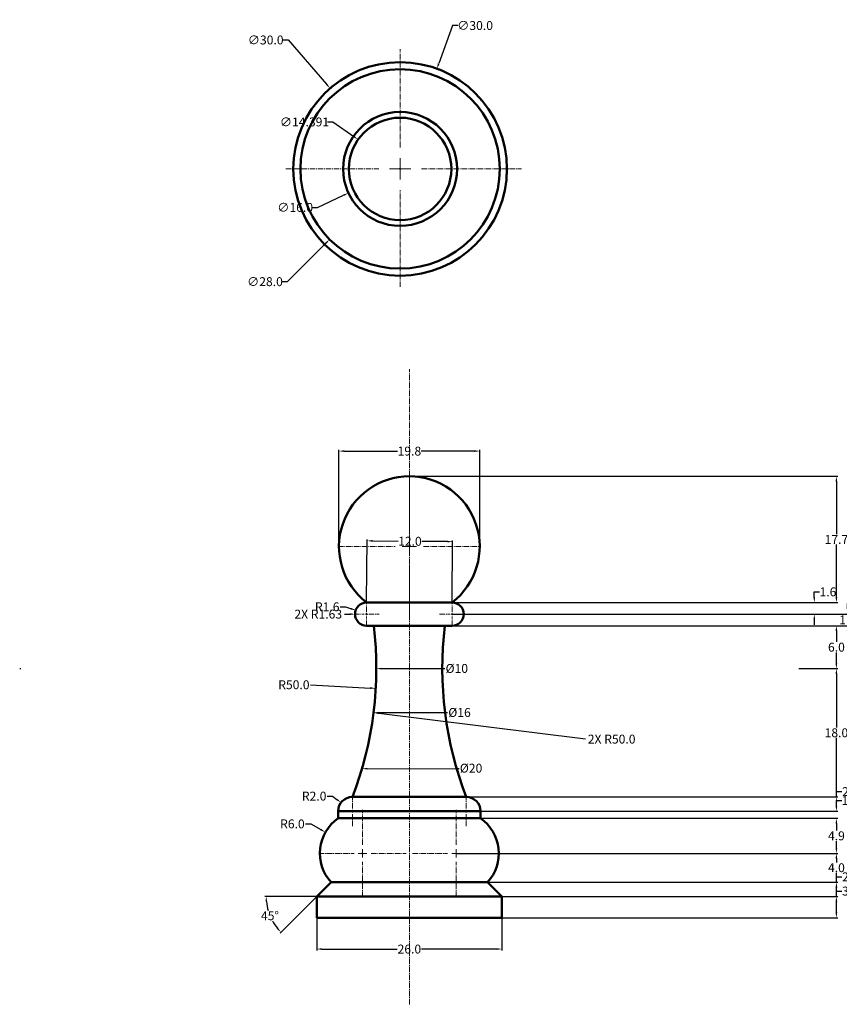
# Model space of a CAD drawing. Units: millimetres. Extents: x 10 to 184, y 6 to 153.
# Tile 1 of 2: x 10 to 125, y 14 to 153. Entities that reach past the tile are written whole.
import ezdxf
from ezdxf import colors
from ezdxf.entities.mleader import LeaderData, LeaderLine
from ezdxf.math import Vec2, Vec3

# ---------------------------------------------------------------- set-up
doc = ezdxf.new("R2010")
doc.units = ezdxf.units.MM
doc.header["$MEASUREMENT"] = 0
doc.linetypes.add('CENTER2', pattern=[1.125, 0.75, -0.125, 0.125, -0.125])
for name, color, linetype, lineweight in [('M-CNTR', 4, 'CENTER2', 18), ('M-DIMS', 2, 'Continuous', 25), ('M-OUTL', 7, 'Continuous', 50)]:
    doc.layers.add(name, color=color, linetype=linetype, lineweight=lineweight)
doc.styles.get("Standard").update_dxf_attribs({"font": 'arial.ttf'})
doc.dimstyles.get("Standard").update_dxf_attribs({"dimtxt": 1.25, "dimasz": 0.75, "dimexe": 0.18, "dimexo": 0.0625, "dimgap": 0.09, "dimtad": 0, "dimtih": 1, "dimtoh": 1, "dimdec": 1, "dimzin": 0, "dimdsep": 46, "dimtxsty": 'Standard', "dimcen": 0.09, "dimadec": 0, "dimazin": 0, "dimtfac": 1, "dimtdec": 1, "dimtofl": 0, "dimtmove": 0, "dimatfit": 3, "dimfxl": 1, "dimtolj": 1, "dimtzin": 0, "dimarcsym": 0})

# ---------------------------------------------------------------- blocks, each defined once
blk = doc.blocks.new('*U1')
at = {"layer": 'M-CNTR', "color": 0, "transparency": 16777216}
blk.add_line((0, -13.67), (0, 75.58), dxfattribs=at)
blk = doc.blocks.new('*U2')
at = {"layer": 'M-CNTR', "color": 0, "transparency": 16777216}
for p, q in [((0, 1.98), (0, 10)), ((-10, 0), (-1.98, 0)), ((1.98, 0), (10, 0)), ((0, -10), (0, -1.98))]:
    blk.add_line(p, q, dxfattribs=at)
at = {"layer": 'M-CNTR', "color": 0, "linetype": 'Continuous', "transparency": 16777216}
for p, q in [((-0.99, 0), (0.99, 0)), ((0, -0.99), (0, 0.99))]:
    blk.add_line(p, q, dxfattribs=at)
blk = doc.blocks.new('*U3')
at = {"layer": 'M-CNTR', "color": 0, "transparency": 16777216}
for p, q in [((0, 1.2), (0, 6.12)), ((-6.12, 0), (-1.2, 0)), ((1.2, 0), (6.12, 0)), ((0, -6.12), (0, -1.2))]:
    blk.add_line(p, q, dxfattribs=at)
at = {"layer": 'M-CNTR', "color": 0, "linetype": 'Continuous', "transparency": 16777216}
for p, q in [((-0.6, 0), (0.6, 0)), ((0, -0.6), (0, 0.6))]:
    blk.add_line(p, q, dxfattribs=at)
blk = doc.blocks.new('*U4')
at = {"layer": 'M-CNTR', "color": 0, "transparency": 16777216}
for p, q in [((0, 1.2), (0, 6.12)), ((-6.12, 0), (-1.2, 0)), ((1.2, 0), (6.12, 0)), ((0, -6.12), (0, -1.2))]:
    blk.add_line(p, q, dxfattribs=at)
at = {"layer": 'M-CNTR', "color": 0, "linetype": 'Continuous', "transparency": 16777216}
for p, q in [((-0.6, 0), (0.6, 0)), ((0, -0.6), (0, 0.6))]:
    blk.add_line(p, q, dxfattribs=at)
blk = doc.blocks.new('*U5')
at = {"layer": 'M-CNTR', "color": 0, "transparency": 16777216}
for p, q in [((0, 0.326), (0, 1.75)), ((-1.75, 0), (-0.326, 0)), ((0.326, 0), (1.75, 0)), ((0, -1.75), (0, -0.326))]:
    blk.add_line(p, q, dxfattribs=at)
at = {"layer": 'M-CNTR', "color": 0, "linetype": 'Continuous', "transparency": 16777216}
for p, q in [((-0.163, 0), (0.163, 0)), ((0, -0.163), (0, 0.163))]:
    blk.add_line(p, q, dxfattribs=at)
blk = doc.blocks.new('*U6')
at = {"layer": 'M-CNTR', "color": 0, "transparency": 16777216}
for p, q in [((0, 0.326), (0, 1.75)), ((-1.75, 0), (-0.326, 0)), ((0.326, 0), (1.75, 0)), ((0, -1.75), (0, -0.326))]:
    blk.add_line(p, q, dxfattribs=at)
at = {"layer": 'M-CNTR', "color": 0, "linetype": 'Continuous', "transparency": 16777216}
for p, q in [((-0.163, 0), (0.163, 0)), ((0, -0.163), (0, 0.163))]:
    blk.add_line(p, q, dxfattribs=at)
blk = doc.blocks.new('*U7')
at = {"layer": 'M-CNTR', "color": 0, "transparency": 16777216}
for p, q in [((0, 0.4), (0, 2.12)), ((-2.12, 0), (-0.4, 0)), ((0.4, 0), (2.12, 0)), ((0, -2.12), (0, -0.4))]:
    blk.add_line(p, q, dxfattribs=at)
at = {"layer": 'M-CNTR', "color": 0, "linetype": 'Continuous', "transparency": 16777216}
for p, q in [((-0.2, 0), (0.2, 0)), ((0, -0.2), (0, 0.2))]:
    blk.add_line(p, q, dxfattribs=at)
blk = doc.blocks.new('*U8')
at = {"layer": 'M-CNTR', "color": 0, "transparency": 16777216}
for p, q in [((0, 0.4), (0, 2.12)), ((-2.12, 0), (-0.4, 0)), ((0.4, 0), (2.12, 0)), ((0, -2.12), (0, -0.4))]:
    blk.add_line(p, q, dxfattribs=at)
at = {"layer": 'M-CNTR', "color": 0, "linetype": 'Continuous', "transparency": 16777216}
for p, q in [((-0.2, 0), (0.2, 0)), ((0, -0.2), (0, 0.2))]:
    blk.add_line(p, q, dxfattribs=at)
blk = doc.blocks.new('*D9')
at = {"layer": 'Defpoints', "color": 0, "transparency": 16777216}
for p in [(78.01, 29.56), (124.99, 29.56), (78.01, 26.56)]:
    blk.add_point(p, dxfattribs=at)
at = {"layer": 'M-DIMS', "color": 0, "lineweight": -2, "transparency": 16777216}
for p, q in [((78.07, 29.56), (125.17, 29.56)), ((124.99, 29.56), (124.99, 30.31)), ((124.99, 30.31), (125.74, 30.31)), ((124.99, 27.31), (124.99, 28.81)), ((78.07, 26.56), (125.17, 26.56))]:
    blk.add_line(p, q, dxfattribs=at)
at = {"layer": 'M-DIMS', "color": 0, "transparency": 16777216}
for points in [[(124.86, 28.81), (125.11, 28.81), (124.99, 29.56)], [(124.86, 27.31), (125.11, 27.31), (124.99, 26.56)]]:
    blk.add_solid(points, dxfattribs=at)
at = {"layer": 'M-DIMS', "color": 0, "transparency": 16777216, "insert": (126.96, 30.31), "char_height": 1.25, "attachment_point": 5}
blk.add_mtext('\\A1;3.0', dxfattribs=at)
blk = doc.blocks.new('*D10')
at = {"layer": 'Defpoints', "color": 0, "transparency": 16777216}
for p in [(76.01, 31.56), (124.99, 31.56), (78.01, 29.56)]:
    blk.add_point(p, dxfattribs=at)
at = {"layer": 'M-DIMS', "color": 0, "lineweight": -2, "transparency": 16777216}
for p, q in [((124.99, 31.56), (124.99, 32.31)), ((124.99, 32.31), (125.74, 32.31)), ((76.07, 31.56), (125.17, 31.56)), ((124.99, 30.31), (124.99, 30.81)), ((78.07, 29.56), (125.17, 29.56))]:
    blk.add_line(p, q, dxfattribs=at)
at = {"layer": 'M-DIMS', "color": 0, "transparency": 16777216}
for points in [[(124.86, 30.81), (125.11, 30.81), (124.99, 31.56)], [(124.86, 30.31), (125.11, 30.31), (124.99, 29.56)]]:
    blk.add_solid(points, dxfattribs=at)
at = {"layer": 'M-DIMS', "color": 0, "transparency": 16777216, "insert": (126.98, 32.31), "char_height": 1.25, "attachment_point": 5}
blk.add_mtext('\\A1;2.0', dxfattribs=at)
blk = doc.blocks.new('*D11')
at = {"layer": 'Defpoints', "color": 0, "transparency": 16777216}
for p in [(71.58, 35.61), (124.99, 35.61), (76.01, 31.56)]:
    blk.add_point(p, dxfattribs=at)
at = {"layer": 'M-DIMS', "color": 0, "lineweight": -2, "transparency": 16777216}
for p, q in [((71.64, 35.61), (125.17, 35.61)), ((124.99, 34.86), (124.99, 34.31)), ((124.99, 32.31), (124.99, 32.86)), ((76.07, 31.56), (125.17, 31.56))]:
    blk.add_line(p, q, dxfattribs=at)
at = {"layer": 'M-DIMS', "color": 0, "transparency": 16777216}
for points in [[(124.86, 34.86), (125.11, 34.86), (124.99, 35.61)], [(124.86, 32.31), (125.11, 32.31), (124.99, 31.56)]]:
    blk.add_solid(points, dxfattribs=at)
at = {"layer": 'M-DIMS', "color": 0, "transparency": 16777216, "insert": (124.99, 33.59), "char_height": 1.25, "attachment_point": 5}
blk.add_mtext('\\A1;4.0', dxfattribs=at)
blk = doc.blocks.new('*D12')
at = {"layer": 'Defpoints', "color": 0, "transparency": 16777216}
for p in [(75.01, 40.53), (124.99, 40.53), (71.58, 35.61)]:
    blk.add_point(p, dxfattribs=at)
at = {"layer": 'M-DIMS', "color": 0, "lineweight": -2, "transparency": 16777216}
for p, q in [((75.07, 40.53), (125.17, 40.53)), ((124.99, 39.78), (124.99, 38.8)), ((124.99, 36.36), (124.99, 37.34)), ((71.64, 35.61), (125.17, 35.61))]:
    blk.add_line(p, q, dxfattribs=at)
at = {"layer": 'M-DIMS', "color": 0, "transparency": 16777216}
for points in [[(124.86, 39.78), (125.11, 39.78), (124.99, 40.53)], [(124.86, 36.36), (125.11, 36.36), (124.99, 35.61)]]:
    blk.add_solid(points, dxfattribs=at)
at = {"layer": 'M-DIMS', "color": 0, "transparency": 16777216, "insert": (124.99, 38.07), "char_height": 1.25, "attachment_point": 5}
blk.add_mtext('\\A1;4.9', dxfattribs=at)
blk = doc.blocks.new('*D13')
at = {"layer": 'Defpoints', "color": 0, "transparency": 16777216}
for p in [(75.01, 41.53), (124.99, 41.53), (75.01, 40.53)]:
    blk.add_point(p, dxfattribs=at)
at = {"layer": 'M-DIMS', "color": 0, "lineweight": -2, "transparency": 16777216}
for p, q in [((124.99, 42.28), (124.99, 43.03)), ((124.99, 43.03), (125.74, 43.03)), ((75.07, 41.53), (125.17, 41.53)), ((75.07, 40.53), (125.17, 40.53)), ((124.99, 39.78), (124.99, 39.03))]:
    blk.add_line(p, q, dxfattribs=at)
at = {"layer": 'M-DIMS', "color": 0, "transparency": 16777216}
for points in [[(124.86, 42.28), (125.11, 42.28), (124.99, 41.53)], [(124.86, 39.78), (125.11, 39.78), (124.99, 40.53)]]:
    blk.add_solid(points, dxfattribs=at)
at = {"layer": 'M-DIMS', "color": 0, "transparency": 16777216, "insert": (126.91, 43.03), "char_height": 1.25, "attachment_point": 5}
blk.add_mtext('\\A1;1.0', dxfattribs=at)
blk = doc.blocks.new('*D14')
at = {"layer": 'Defpoints', "color": 0, "transparency": 16777216}
for p in [(73.01, 43.53), (124.99, 43.53), (75.01, 41.53)]:
    blk.add_point(p, dxfattribs=at)
at = {"layer": 'M-DIMS', "color": 0, "lineweight": -2, "transparency": 16777216}
for p, q in [((124.99, 43.53), (124.99, 44.28)), ((124.99, 44.28), (125.74, 44.28)), ((73.07, 43.53), (125.17, 43.53)), ((75.07, 41.53), (125.17, 41.53)), ((124.99, 42.28), (124.99, 42.78))]:
    blk.add_line(p, q, dxfattribs=at)
at = {"layer": 'M-DIMS', "color": 0, "transparency": 16777216}
for points in [[(124.86, 42.78), (125.11, 42.78), (124.99, 43.53)], [(124.86, 42.28), (125.11, 42.28), (124.99, 41.53)]]:
    blk.add_solid(points, dxfattribs=at)
at = {"layer": 'M-DIMS', "color": 0, "transparency": 16777216, "insert": (126.98, 44.28), "char_height": 1.25, "attachment_point": 5}
blk.add_mtext('\\A1;2.0', dxfattribs=at)
blk = doc.blocks.new('*D15')
at = {"layer": 'Defpoints', "color": 0, "transparency": 16777216}
for p in [(119.64, 61.56), (124.99, 61.56), (73.01, 43.53)]:
    blk.add_point(p, dxfattribs=at)
at = {"layer": 'M-DIMS', "color": 0, "lineweight": -2, "transparency": 16777216}
for p, q in [((119.7, 61.56), (125.17, 61.56)), ((124.99, 60.81), (124.99, 53.28)), ((124.99, 44.28), (124.99, 51.82)), ((73.07, 43.53), (125.17, 43.53))]:
    blk.add_line(p, q, dxfattribs=at)
at = {"layer": 'M-DIMS', "color": 0, "transparency": 16777216}
for points in [[(124.86, 60.81), (125.11, 60.81), (124.99, 61.56)], [(124.86, 44.28), (125.11, 44.28), (124.99, 43.53)]]:
    blk.add_solid(points, dxfattribs=at)
at = {"layer": 'M-DIMS', "color": 0, "transparency": 16777216, "insert": (124.99, 52.55), "char_height": 1.25, "attachment_point": 5}
blk.add_mtext('\\A1;18.0', dxfattribs=at)
blk = doc.blocks.new('*D16')
at = {"layer": 'Defpoints', "color": 0, "transparency": 16777216}
for p in [(71.01, 67.59), (124.99, 67.59), (119.64, 61.56)]:
    blk.add_point(p, dxfattribs=at)
at = {"layer": 'M-DIMS', "color": 0, "lineweight": -2, "transparency": 16777216}
for p, q in [((71.07, 67.59), (125.17, 67.59)), ((124.99, 66.84), (124.99, 65.31)), ((124.99, 62.31), (124.99, 63.85)), ((119.7, 61.56), (125.17, 61.56))]:
    blk.add_line(p, q, dxfattribs=at)
at = {"layer": 'M-DIMS', "color": 0, "transparency": 16777216}
for points in [[(124.86, 66.84), (125.11, 66.84), (124.99, 67.59)], [(124.86, 62.31), (125.11, 62.31), (124.99, 61.56)]]:
    blk.add_solid(points, dxfattribs=at)
at = {"layer": 'M-DIMS', "color": 0, "transparency": 16777216, "insert": (124.99, 64.58), "char_height": 1.25, "attachment_point": 5}
blk.add_mtext('\\A1;6.0', dxfattribs=at)
blk = doc.blocks.new('*D17')
at = {"layer": 'Defpoints', "color": 0, "transparency": 16777216}
for p in [(71.01, 69.22), (126.56, 69.22), (71.01, 67.59)]:
    blk.add_point(p, dxfattribs=at)
at = {"layer": 'M-DIMS', "color": 0, "lineweight": -2, "transparency": 16777216}
for p, q in [((126.56, 69.97), (126.56, 70.72)), ((71.07, 69.22), (126.74, 69.22)), ((71.07, 67.59), (126.74, 67.59)), ((126.56, 66.84), (126.56, 66.09))]:
    blk.add_line(p, q, dxfattribs=at)
at = {"layer": 'M-DIMS', "color": 0, "transparency": 16777216}
for points in [[(126.44, 69.97), (126.69, 69.97), (126.56, 69.22)], [(126.44, 66.84), (126.69, 66.84), (126.56, 67.59)]]:
    blk.add_solid(points, dxfattribs=at)
at = {"layer": 'M-DIMS', "color": 0, "transparency": 16777216, "insert": (126.56, 68.41), "char_height": 1.25, "attachment_point": 5}
blk.add_mtext('\\A1;1.6', dxfattribs=at)
blk = doc.blocks.new('*D18')
at = {"layer": 'Defpoints', "color": 0, "transparency": 16777216}
for p in [(71.01, 70.85), (121.88, 70.85), (71.01, 69.22)]:
    blk.add_point(p, dxfattribs=at)
at = {"layer": 'M-DIMS', "color": 0, "lineweight": -2, "transparency": 16777216}
for p, q in [((121.88, 71.6), (121.88, 72.35)), ((121.88, 72.35), (122.63, 72.35)), ((71.07, 70.85), (122.06, 70.85)), ((71.07, 69.22), (122.06, 69.22)), ((121.88, 68.47), (121.88, 67.72))]:
    blk.add_line(p, q, dxfattribs=at)
at = {"layer": 'M-DIMS', "color": 0, "transparency": 16777216}
for points in [[(121.76, 71.6), (122.01, 71.6), (121.88, 70.85)], [(121.76, 68.47), (122.01, 68.47), (121.88, 69.22)]]:
    blk.add_solid(points, dxfattribs=at)
at = {"layer": 'M-DIMS', "color": 0, "transparency": 16777216, "insert": (123.8, 72.35), "char_height": 1.25, "attachment_point": 5}
blk.add_mtext('\\A1;1.6', dxfattribs=at)
blk = doc.blocks.new('*D19')
at = {"layer": 'Defpoints', "color": 0, "transparency": 16777216}
for p in [(65.01, 88.59), (124.99, 88.59), (71.01, 70.85)]:
    blk.add_point(p, dxfattribs=at)
at = {"layer": 'M-DIMS', "color": 0, "lineweight": -2, "transparency": 16777216}
for p, q in [((65.07, 88.59), (125.17, 88.59)), ((124.99, 87.84), (124.99, 80.44)), ((124.99, 71.6), (124.99, 79)), ((71.07, 70.85), (125.17, 70.85))]:
    blk.add_line(p, q, dxfattribs=at)
at = {"layer": 'M-DIMS', "color": 0, "transparency": 16777216}
for points in [[(124.86, 87.84), (125.11, 87.84), (124.99, 88.59)], [(124.86, 71.6), (125.11, 71.6), (124.99, 70.85)]]:
    blk.add_solid(points, dxfattribs=at)
at = {"layer": 'M-DIMS', "color": 0, "transparency": 16777216, "insert": (124.99, 79.72), "char_height": 1.25, "attachment_point": 5}
blk.add_mtext('\\A1;17.7', dxfattribs=at)
blk = doc.blocks.new('*D20')
at = {"layer": 'Defpoints', "color": 0, "transparency": 16777216}
for p in [(52.01, 26.56), (78.01, 26.56), (78.01, 22.16)]:
    blk.add_point(p, dxfattribs=at)
at = {"layer": 'M-DIMS', "color": 0, "lineweight": -2, "transparency": 16777216}
for p, q in [((52.01, 26.5), (52.01, 21.98)), ((78.01, 26.5), (78.01, 21.98)), ((52.76, 22.16), (63.28, 22.16)), ((77.26, 22.16), (66.73, 22.16))]:
    blk.add_line(p, q, dxfattribs=at)
at = {"layer": 'M-DIMS', "color": 0, "transparency": 16777216}
for points in [[(52.76, 22.29), (52.76, 22.04), (52.01, 22.16)], [(77.26, 22.29), (77.26, 22.04), (78.01, 22.16)]]:
    blk.add_solid(points, dxfattribs=at)
at = {"layer": 'M-DIMS', "color": 0, "transparency": 16777216, "insert": (65.01, 22.16), "char_height": 1.25, "attachment_point": 5}
blk.add_mtext('\\A1;26.0', dxfattribs=at)
blk = doc.blocks.new('*D21')
at = {"layer": 'Defpoints', "color": 0, "transparency": 16777216}
for p in [(55.41, 42.74), (57.01, 41.53)]:
    blk.add_point(p, dxfattribs=at)
at = {"layer": 'M-DIMS', "color": 0, "lineweight": -2, "transparency": 16777216}
for p, q in [((53.47, 43.65), (54.22, 43.65)), ((54.22, 43.65), (54.81, 43.19)), ((56.92, 41.53), (57.1, 41.53)), ((57.01, 41.44), (57.01, 41.62))]:
    blk.add_line(p, q, dxfattribs=at)
at = {"layer": 'M-DIMS', "color": 0, "transparency": 16777216}
blk.add_solid([(54.89, 43.29), (54.74, 43.09), (55.41, 42.74)], dxfattribs=at)
at = {"layer": 'M-DIMS', "color": 0, "transparency": 16777216, "insert": (51.64, 43.65), "char_height": 1.25, "attachment_point": 5}
blk.add_mtext('\\A1;R2.0', dxfattribs=at)
blk = doc.blocks.new('*D22')
at = {"layer": 'Defpoints', "color": 0, "transparency": 16777216}
for p in [(53.22, 38.57), (58.44, 35.61)]:
    blk.add_point(p, dxfattribs=at)
at = {"layer": 'M-DIMS', "color": 0, "lineweight": -2, "transparency": 16777216}
for p, q in [((50.4, 39.75), (51.15, 39.75)), ((51.15, 39.75), (52.57, 38.94)), ((58.35, 35.61), (58.53, 35.61)), ((58.44, 35.52), (58.44, 35.7))]:
    blk.add_line(p, q, dxfattribs=at)
at = {"layer": 'M-DIMS', "color": 0, "transparency": 16777216}
blk.add_solid([(52.63, 39.05), (52.51, 38.84), (53.22, 38.57)], dxfattribs=at)
at = {"layer": 'M-DIMS', "color": 0, "transparency": 16777216, "insert": (48.58, 39.75), "char_height": 1.25, "attachment_point": 5}
blk.add_mtext('\\A1;R6.0', dxfattribs=at)
blk = doc.blocks.new('*D23')
at = {"layer": 'Defpoints', "color": 0, "transparency": 16777216}
for p in [(57.47, 69.76), (59.01, 69.22)]:
    blk.add_point(p, dxfattribs=at)
at = {"layer": 'M-DIMS', "color": 0, "lineweight": -2, "transparency": 16777216}
for p, q in [((55.3, 70.25), (56.05, 70.25)), ((56.05, 70.25), (56.76, 70)), ((58.92, 69.22), (59.1, 69.22)), ((59.01, 69.13), (59.01, 69.31))]:
    blk.add_line(p, q, dxfattribs=at)
at = {"layer": 'M-DIMS', "color": 0, "transparency": 16777216}
blk.add_solid([(56.8, 70.12), (56.72, 69.88), (57.47, 69.76)], dxfattribs=at)
at = {"layer": 'M-DIMS', "color": 0, "transparency": 16777216, "insert": (53.47, 70.25), "char_height": 1.25, "attachment_point": 5}
blk.add_mtext('\\A1;R1.6', dxfattribs=at)
blk = doc.blocks.new('*D24')
at = {"layer": 'Defpoints', "color": 0, "transparency": 16777216}
for p in [(71.09, 79.4), (59.01, 70.97), (71.01, 70.85)]:
    blk.add_point(p, dxfattribs=at)
at = {"layer": 'M-DIMS', "color": 0, "lineweight": -2, "transparency": 16777216}
for p, q in [((59.01, 71.03), (59.09, 79.7)), ((59.84, 79.52), (63.44, 79.48)), ((70.34, 79.41), (66.74, 79.45)), ((71.01, 70.91), (71.09, 79.58))]:
    blk.add_line(p, q, dxfattribs=at)
at = {"layer": 'M-DIMS', "color": 0, "transparency": 16777216}
for points in [[(59.84, 79.64), (59.84, 79.39), (59.09, 79.52)], [(70.34, 79.54), (70.34, 79.29), (71.09, 79.4)]]:
    blk.add_solid(points, dxfattribs=at)
at = {"layer": 'M-DIMS', "color": 0, "transparency": 16777216, "insert": (65.09, 79.46), "char_height": 1.25, "attachment_point": 5}
blk.add_mtext('\\A1;12.0', dxfattribs=at)
blk = doc.blocks.new('*D25')
at = {"layer": 'Defpoints', "color": 0, "transparency": 16777216}
for p in [(74.89, 92.13), (55.12, 78.71), (74.89, 78.71)]:
    blk.add_point(p, dxfattribs=at)
at = {"layer": 'M-DIMS', "color": 0, "lineweight": -2, "transparency": 16777216}
for p, q in [((55.12, 78.77), (55.12, 92.31)), ((55.87, 92.13), (63.35, 92.13)), ((74.14, 92.13), (66.66, 92.13)), ((74.89, 78.77), (74.89, 92.31))]:
    blk.add_line(p, q, dxfattribs=at)
at = {"layer": 'M-DIMS', "color": 0, "transparency": 16777216}
for points in [[(55.87, 92.26), (55.87, 92.01), (55.12, 92.13)], [(74.14, 92.26), (74.14, 92.01), (74.89, 92.13)]]:
    blk.add_solid(points, dxfattribs=at)
at = {"layer": 'M-DIMS', "color": 0, "transparency": 16777216, "insert": (65.01, 92.13), "char_height": 1.25, "attachment_point": 5}
blk.add_mtext('\\A1;19.8', dxfattribs=at)
blk = doc.blocks.new('*D26')
at = {"layer": 'Defpoints', "color": 0, "transparency": 16777216}
for p in [(54.01, 31.56), (52.01, 29.56), (52.01, 29.56), (78.01, 29.56), (45.13, 27.72)]:
    blk.add_point(p, dxfattribs=at)
at = {"layer": 'M-DIMS', "color": 0, "lineweight": -2, "transparency": 16777216}
for p, q in [((51.94, 29.56), (44.71, 29.56)), ((51.96, 29.52), (46.84, 24.4))]:
    blk.add_line(p, q, dxfattribs=at)
for start, end in [(186.0378, 196.3063), (208.9859, 218.9622)]:
    blk.add_arc((52.01, 29.56), 7.12, start, end, dxfattribs=at)
at = {"layer": 'M-DIMS', "color": 0, "transparency": 16777216}
for points in [[(44.8, 28.81), (45.05, 28.82), (44.89, 29.56)], [(46.56, 25.17), (46.38, 25), (46.97, 24.53)]]:
    blk.add_solid(points, dxfattribs=at)
at = {"layer": 'M-DIMS', "color": 0, "transparency": 16777216, "insert": (45.43, 26.84), "char_height": 1.25, "attachment_point": 5}
blk.add_mtext('\\A1;45°', dxfattribs=at)
blk = doc.blocks.new('*D27')
at = {"layer": 'Defpoints', "color": 0, "transparency": 16777216}
for p in [(10.37, 61.56), (60.29, 58.79)]:
    blk.add_point(p, dxfattribs=at)
at = {"layer": 'M-DIMS', "color": 0, "lineweight": -2, "transparency": 16777216}
blk.add_line((51.1, 59.3), (59.54, 58.83), dxfattribs=at)
at = {"layer": 'M-DIMS', "color": 0, "transparency": 16777216}
blk.add_solid([(59.55, 58.96), (59.54, 58.71), (60.29, 58.79)], dxfattribs=at)
at = {"layer": 'M-DIMS', "color": 0, "transparency": 16777216, "insert": (48.79, 59.3), "char_height": 1.25, "attachment_point": 5}
blk.add_mtext('\\A1;R50.0', dxfattribs=at)
blk = doc.blocks.new('*U28')
at = {"layer": 'M-CNTR', "color": 0, "transparency": 16777216}
for p, q in [((0, 3), (0, 16.83)), ((-16.06, 0), (-3, 0)), ((3, 0), (17.06, 0)), ((0, -16.56), (0, -3))]:
    blk.add_line(p, q, dxfattribs=at)
at = {"layer": 'M-CNTR', "color": 0, "linetype": 'Continuous', "transparency": 16777216}
for p, q in [((0, -1.5), (0, 1.5)), ((-1.5, 0), (1.5, 0))]:
    blk.add_line(p, q, dxfattribs=at)
blk = doc.blocks.new('*D29')
at = {"layer": 'Defpoints', "color": 0, "transparency": 16777216}
for p in [(68.87, 145.86), (58.55, 117.7)]:
    blk.add_point(p, dxfattribs=at)
at = {"layer": 'M-DIMS', "color": 0, "lineweight": -2, "transparency": 16777216}
for p, q in [((71.09, 151.93), (69.13, 146.57)), ((71.84, 151.93), (71.09, 151.93)), ((63.62, 131.78), (63.8, 131.78)), ((63.71, 131.69), (63.71, 131.87))]:
    blk.add_line(p, q, dxfattribs=at)
at = {"layer": 'M-DIMS', "color": 0, "transparency": 16777216}
blk.add_solid([(69.01, 146.61), (69.25, 146.52), (68.87, 145.86)], dxfattribs=at)
at = {"layer": 'M-DIMS', "color": 0, "transparency": 16777216, "insert": (74.24, 151.93), "char_height": 1.25, "attachment_point": 5}
blk.add_mtext('\\A1;∅30.0', dxfattribs=at)
blk = doc.blocks.new('PAWN-ELEVATION')
for p, q in [((13, 44.29), (7, 44.29)), ((13, 44.29), (19, 44.29)), ((13, 41.03), (7, 41.03)), ((13, 41.03), (8, 41.03)), ((13, 41.03), (19, 41.03)), ((5, 16.97), (21, 16.97)), ((3, 13.97), (3, 14.97)), ((3, 14.97), (23, 14.97)), ((3, 13.97), (23, 13.97)), ((23, 14.97), (23, 13.97)), ((0, 3), (2, 5)), ((2, 5), (24, 5)), ((26, 3), (24, 5)), ((26, 3), (0, 3)), ((0, 3), (0, 0)), ((26, 0), (26, 3)), ((0, 0), (26, 0))]:
    blk.add_line(p, q)
for centre, radius, start, end in [((13, 52.15), 9.88, 307.3742, 232.6258), ((7, 42.66), 1.63, 90, 270), ((19, 42.66), 1.63, 270, 90), ((-41.64, 35), 50, 338.8606, 6.9245), ((67.63, 35), 50, 173.0755, 201.1394), ((5, 14.97), 2, 90, 180), ((21, 14.97), 2, 360, 90), ((6.43, 9.05), 6, 124.8635, 222.4141), ((19.57, 9.05), 6, 317.5859, 55.1365)]:
    blk.add_arc(centre, radius, start, end)
blk = doc.blocks.new('*D33')
at = {"layer": 'Defpoints', "color": 0, "transparency": 16777216}
for p in [(53.87, 143.11), (73.54, 120.45)]:
    blk.add_point(p, dxfattribs=at)
at = {"layer": 'M-DIMS', "color": 0, "lineweight": -2, "transparency": 16777216}
for p, q in [((47.22, 149.9), (47.97, 149.9)), ((47.97, 149.9), (53.38, 143.67)), ((63.62, 131.78), (63.8, 131.78)), ((63.71, 131.69), (63.71, 131.87))]:
    blk.add_line(p, q, dxfattribs=at)
at = {"layer": 'M-DIMS', "color": 0, "transparency": 16777216}
blk.add_solid([(53.48, 143.75), (53.29, 143.59), (53.87, 143.11)], dxfattribs=at)
at = {"layer": 'M-DIMS', "color": 0, "transparency": 16777216, "insert": (44.83, 149.9), "char_height": 1.25, "attachment_point": 5}
blk.add_mtext('\\A1;∅30.0', dxfattribs=at)
blk = doc.blocks.new('*D34')
at = {"layer": 'Defpoints', "color": 0, "transparency": 16777216}
for p in [(73.61, 141.68), (53.81, 121.88)]:
    blk.add_point(p, dxfattribs=at)
at = {"layer": 'M-DIMS', "color": 0, "lineweight": -2, "transparency": 16777216}
for p, q in [((63.62, 131.78), (63.8, 131.78)), ((63.71, 131.69), (63.71, 131.87)), ((47.87, 115.94), (53.28, 121.35)), ((47.12, 115.94), (47.87, 115.94))]:
    blk.add_line(p, q, dxfattribs=at)
at = {"layer": 'M-DIMS', "color": 0, "transparency": 16777216}
blk.add_solid([(53.19, 121.44), (53.37, 121.26), (53.81, 121.88)], dxfattribs=at)
at = {"layer": 'M-DIMS', "color": 0, "transparency": 16777216, "insert": (44.73, 115.94), "char_height": 1.25, "attachment_point": 5}
blk.add_mtext('\\A1;∅28.0', dxfattribs=at)
blk = doc.blocks.new('*D35')
at = {"layer": 'Defpoints', "color": 0, "transparency": 16777216}
for p in [(70.96, 135.16), (56.46, 128.4)]:
    blk.add_point(p, dxfattribs=at)
at = {"layer": 'M-DIMS', "color": 0, "lineweight": -2, "transparency": 16777216}
for p, q in [((63.62, 131.78), (63.8, 131.78)), ((63.71, 131.69), (63.71, 131.87)), ((52.11, 126.37), (55.78, 128.08)), ((51.36, 126.37), (52.11, 126.37))]:
    blk.add_line(p, q, dxfattribs=at)
at = {"layer": 'M-DIMS', "color": 0, "transparency": 16777216}
blk.add_solid([(55.73, 128.19), (55.83, 127.97), (56.46, 128.4)], dxfattribs=at)
at = {"layer": 'M-DIMS', "color": 0, "transparency": 16777216, "insert": (48.97, 126.37), "char_height": 1.25, "attachment_point": 5}
blk.add_mtext('\\A1;∅16.0', dxfattribs=at)
blk = doc.blocks.new('*D36')
at = {"layer": 'Defpoints', "color": 0, "transparency": 16777216}
for p in [(57.81, 135.91), (69.6, 127.65)]:
    blk.add_point(p, dxfattribs=at)
at = {"layer": 'M-DIMS', "color": 0, "lineweight": -2, "transparency": 16777216}
for p, q in [((53.53, 138.38), (54.28, 138.38)), ((54.28, 138.38), (57.2, 136.34)), ((63.62, 131.78), (63.8, 131.78)), ((63.71, 131.69), (63.71, 131.87))]:
    blk.add_line(p, q, dxfattribs=at)
at = {"layer": 'M-DIMS', "color": 0, "transparency": 16777216}
blk.add_solid([(57.27, 136.44), (57.13, 136.23), (57.81, 135.91)], dxfattribs=at)
at = {"layer": 'M-DIMS', "color": 0, "transparency": 16777216, "insert": (50.28, 138.38), "char_height": 1.25, "attachment_point": 5}
blk.add_mtext('\\A1;∅14.391', dxfattribs=at)
blk = doc.blocks.new('*D37')
at = {"layer": 'Defpoints', "color": 0, "transparency": 16777216}
for p in [(10.37, 61.56), (59.99, 55.38)]:
    blk.add_point(p, dxfattribs=at)
at = {"layer": 'M-DIMS', "color": 0, "lineweight": -2, "transparency": 16777216}
for p, q in [((10.28, 61.56), (10.46, 61.56)), ((10.37, 61.47), (10.37, 61.65)), ((89.76, 51.66), (60.73, 55.28))]:
    blk.add_line(p, q, dxfattribs=at)
at = {"layer": 'M-DIMS', "color": 0, "transparency": 16777216}
blk.add_solid([(60.75, 55.41), (60.71, 55.16), (59.99, 55.38)], dxfattribs=at)
at = {"layer": 'M-DIMS', "color": 0, "transparency": 16777216, "insert": (93.42, 51.66), "char_height": 1.25, "attachment_point": 5}
blk.add_mtext('\\A1;2X R50.0', dxfattribs=at)
blk = doc.blocks.new('*D40')
at = {"layer": 'Defpoints', "color": 0, "transparency": 16777216}
for p in [(57.38, 69.22), (59.01, 69.22)]:
    blk.add_point(p, dxfattribs=at)
at = {"layer": 'M-DIMS', "color": 0, "lineweight": -2, "transparency": 16777216}
for p, q in [((55.88, 69.22), (56.63, 69.22)), ((58.92, 69.22), (59.1, 69.22)), ((59.01, 69.13), (59.01, 69.31))]:
    blk.add_line(p, q, dxfattribs=at)
at = {"layer": 'M-DIMS', "color": 0, "transparency": 16777216}
blk.add_solid([(56.63, 69.35), (56.63, 69.1), (57.38, 69.22)], dxfattribs=at)
at = {"layer": 'M-DIMS', "color": 0, "transparency": 16777216, "insert": (52.21, 69.22), "char_height": 1.25, "attachment_point": 5}
blk.add_mtext('\\A1;2X R1.63', dxfattribs=at)

msp = doc.modelspace()

# ---------------------------------------------------------------- linework, layer by layer
at = {"layer": 'M-OUTL'}
for radius in [15, 14, 8, 7.1957]:
    msp.add_circle((63.7084, 131.7792), radius, dxfattribs=at)

# ---------------------------------------------------------------- block references
at = {"layer": 'M-CNTR'}
for name, p in [('*U28', (63.7084, 131.7792)), ('*U1', (65.0055, 28.0621)), ('*U2', (65.0055, 78.7071)), ('*U6', (59.0055, 69.2221)), ('*U5', (71.0055, 69.2221)), ('*U8', (57.0055, 41.5321)), ('*U7', (73.0055, 41.5321)), ('*U3', (58.4353, 35.609)), ('*U4', (71.5758, 35.609))]:
    msp.add_blockref(name, p, dxfattribs=at)
at = {"layer": 'M-OUTL'}
msp.add_blockref('PAWN-ELEVATION', (52.006, 26.562), dxfattribs=at)

# ---------------------------------------------------------------- dimensions: what is measured, and where the dimension line sits
at = {"layer": 'M-DIMS'}
for p1, p2, override, picture, middle in [((58.5463, 117.6954), (68.8705, 145.863), {"dimclrd": 0, "dimclre": 0, "dimclrt": 0}, '*D29', (74.2351, 151.9286)), ((73.5425, 120.4526), (53.8743, 143.1058), {"dimdec": 1, "dimlfac": 1, "dimrnd": 0, "dimzin": 0, "dimdsep": 46, "dimlunit": 2}, '*D33', (44.8326, 149.9017)), ((73.608, 141.6786), (53.8088, 121.8798), {"dimdec": 1, "dimlfac": 1, "dimrnd": 0, "dimzin": 0, "dimdsep": 46, "dimlunit": 2}, '*D34', (44.7277, 115.9402)), ((69.6026, 127.6516), (57.8143, 135.9068), {"dimdec": 3, "dimlfac": 1, "dimrnd": 0, "dimzin": 0, "dimdsep": 46, "dimlunit": 2}, '*D36', (50.2838, 138.3834)), ((70.9584, 135.1612), (56.4584, 128.3972), {"dimdec": 1, "dimlfac": 1, "dimrnd": 0, "dimzin": 0, "dimdsep": 46, "dimlunit": 2}, '*D35', (48.9671, 126.368))]:
    dim = msp.add_diameter_dim_2p(p1=p1, p2=p2, dimstyle='Standard', override=override, dxfattribs=at)
    dim.commit()
    dim.dimension.update_dxf_attribs({"geometry": picture, "text_midpoint": middle, "dimtype": 163})
for base, p1, p2, picture, middle in [((74.8899, 92.1303), (55.1212, 78.7071), (74.8899, 78.7071), '*D25', (65.0055, 92.1303)), ((78.0055, 22.1624), (52.0055, 26.5621), (78.0055, 26.5621), '*D20', (65.0055, 22.1624))]:
    dim = msp.add_linear_dim(base=base, p1=p1, p2=p2, dimstyle='Standard', override={"dimclrd": 0, "dimclre": 0, "dimclrt": 0}, dxfattribs=at)
    dim.commit()
    dim.dimension.update_dxf_attribs({"geometry": picture, "text_midpoint": middle})
for base, p1, p2, picture, middle in [((124.9896, 88.5914), (71.0055, 70.8521), (65.0055, 88.5914), '*D19', (124.9896, 79.7218)), ((124.9896, 67.5921), (119.6408, 61.564), (71.0055, 67.5921), '*D16', (124.9896, 64.578)), ((124.9896, 61.564), (73.0055, 43.5321), (119.6408, 61.564), '*D15', (124.9896, 52.548)), ((124.9896, 43.5321), (75.0055, 41.5321), (73.0055, 43.5321), '*D14', (126.976, 44.2821)), ((124.9896, 41.5321), (75.0055, 40.5321), (75.0055, 41.5321), '*D13', (126.9065, 43.0321)), ((124.9896, 40.5321), (71.5758, 35.609), (75.0055, 40.5321), '*D12', (124.9896, 38.0705)), ((124.9896, 35.609), (76.0055, 31.5621), (71.5758, 35.609), '*D11', (124.9896, 33.5855)), ((124.9896, 31.5621), (78.0055, 29.5621), (76.0055, 31.5621), '*D10', (126.976, 32.3121)), ((124.9896, 29.5621), (78.0055, 26.5621), (78.0055, 29.5621), '*D9', (126.9649, 30.3121))]:
    dim = msp.add_linear_dim(base=base, p1=p1, p2=p2, angle=270, dimstyle='Standard', override={"dimclrd": 0, "dimclre": 0, "dimclrt": 0}, dxfattribs=at)
    dim.commit()
    dim.dimension.update_dxf_attribs({"geometry": picture, "text_midpoint": middle})
dim = msp.add_aligned_dim(p1=(59.0055, 70.9721), p2=(71.0055, 70.8521), distance=8.553, dimstyle='Standard', override={"dimclrd": 0, "dimclre": 0, "dimclrt": 0}, dxfattribs=at)
dim.commit()
dim.dimension.update_dxf_attribs({"geometry": '*D24', "text_midpoint": (65.0911, 79.4647)})
for base, p1, p2, picture, middle in [((121.881, 70.8521), (71.0055, 69.2221), (71.0055, 70.8521), '*D18', (123.7996, 72.3521)), ((126.561, 69.2221), (71.0055, 67.5921), (71.0055, 69.2221), '*D17', (126.561, 68.4071))]:
    dim = msp.add_linear_dim(base=base, p1=p1, p2=p2, angle=270, dimstyle='Standard', override={"dimclrd": 0, "dimclre": 0, "dimclrt": 0}, dxfattribs=at)
    dim.commit()
    dim.dimension.update_dxf_attribs({"geometry": picture, "text_midpoint": middle, "dimtype": 160})
dim = msp.add_radius_dim(center=(59.0055, 69.2221), mpoint=(57.3755, 69.222), text='2X <>', dimstyle='Standard', override={"dimdec": 2, "dimlfac": 1, "dimrnd": 0, "dimzin": 0, "dimdsep": 46, "dimlunit": 2}, dxfattribs=at)
dim.commit()
dim.dimension.update_dxf_attribs({"geometry": '*D40', "text_midpoint": (52.2103, 69.2219)})
for center, mpoint, picture, middle in [((59.0055, 69.2221), (57.4652, 69.7551), '*D23', (53.472, 70.2456)), ((57.0055, 41.5321), (55.4118, 42.7403), '*D21', (51.6426, 43.6466))]:
    dim = msp.add_radius_dim(center=center, mpoint=mpoint, dimstyle='Standard', override={"dimclrd": 0, "dimclre": 0, "dimclrt": 0}, dxfattribs=at)
    dim.commit()
    dim.dimension.update_dxf_attribs({"geometry": picture, "text_midpoint": middle})
dim = msp.add_radius_dim(center=(10.3702, 61.564), mpoint=(59.986, 55.377), text='2X <>', dimstyle='Standard', override={"dimdec": 1, "dimlfac": 1, "dimrnd": 0, "dimzin": 0, "dimdsep": 46, "dimlunit": 2}, dxfattribs=at)
dim.commit()
dim.dimension.update_dxf_attribs({"geometry": '*D37', "text_midpoint": (89.7554, 51.6648), "dimtype": 164})
for center, mpoint, picture, middle in [((10.3702, 61.564), (60.2932, 58.7887), '*D27', (51.0994, 59.2998)), ((58.4353, 35.609), (53.2188, 38.5736), '*D22', (48.5755, 39.7497))]:
    dim = msp.add_radius_dim(center=center, mpoint=mpoint, dimstyle='Standard', override={"dimclrd": 0, "dimclre": 0, "dimclrt": 0}, dxfattribs=at)
    dim.commit()
    dim.dimension.update_dxf_attribs({"geometry": picture, "text_midpoint": middle, "dimtype": 164})
dim = msp.add_angular_dim_2l(base=(45.1277, 27.7192), line1=((78.0055, 29.5621), (52.0055, 29.5621)), line2=((52.0055, 29.5621), (54.0055, 31.5621)), dimstyle='Standard', override={"dimclrd": 0, "dimclre": 0, "dimclrt": 0}, dxfattribs=at)
dim.commit()
dim.dimension.update_dxf_attribs({"geometry": '*D26', "text_midpoint": (45.4271, 26.8372)})

# ---------------------------------------------------------------- leaders
ml = msp.add_multileader_mtext('Standard', dxfattribs=at)
ml.set_content('%%C10', color=256)
ml.set_leader_properties()
ml.build(insert=Vec2(0, 0))
ml.multileader.update_dxf_attribs({"dogleg_length": 0.36, "arrow_head_size": 0.75})
ctx = ml.context
ctx.base_point, ctx.char_height, ctx.arrow_head_size, ctx.landing_gap_size, ctx.plane_origin = Vec3(70.0008, 61.564), 1.25, 0.75, 0.09, Vec3(60.3702, 61.564)
notes = []
notes.append((ctx, [(0, (1, 1, 0), (69.6408, 61.564), (1, 0), 0.36, [(0, [(60.3702, 61.564)], 0, [])])]))
ctx.mtext.insert, ctx.mtext.width, ctx.mtext.flow_direction = Vec3(70.0908, 62.2141), 0.7946, 5
ml = msp.add_multileader_mtext('Standard', dxfattribs=at)
ml.set_content('%%C16', color=256)
ml.set_leader_properties()
ml.build(insert=Vec2(0, 0))
ml.multileader.update_dxf_attribs({"dogleg_length": 0.36, "arrow_head_size": 0.75})
ctx = ml.context
ctx.base_point, ctx.char_height, ctx.arrow_head_size, ctx.landing_gap_size, ctx.plane_origin = Vec3(70.385, 55.3775), 1.25, 0.75, 0.09, Vec3(59.986, 55.3775)
notes.append((ctx, [(0, (1, 1, 0), (70.025, 55.3775), (1, 0), 0.36, [(0, [(59.986, 55.3775)], 0, [])])]))
ctx.mtext.insert, ctx.mtext.width, ctx.mtext.flow_direction = Vec3(70.475, 56.0276), 0.7946, 5
ml = msp.add_multileader_mtext('Standard', dxfattribs=at)
ml.set_content('%%C20', color=256)
ml.set_leader_properties()
ml.build(insert=Vec2(0, 0))
ml.multileader.update_dxf_attribs({"dogleg_length": 0.36, "arrow_head_size": 0.75})
ctx = ml.context
ctx.base_point, ctx.char_height, ctx.arrow_head_size, ctx.landing_gap_size, ctx.plane_origin = Vec3(72.0047, 47.5508), 1.25, 0.75, 0.09, Vec3(58.352, 47.5014)
notes.append((ctx, [(0, (1, 1, 0), (71.6447, 47.5508), (1, 0), 0.36, [(0, [(58.352, 47.5014)], 0, [])])]))
ctx.mtext.insert, ctx.mtext.width, ctx.mtext.flow_direction = Vec3(72.0947, 48.201), 0.7946, 5
for ctx, leaders in notes:
    for number, flags, end, landing, length, lines in leaders:
        leader = LeaderData()
        leader.index, (leader.has_last_leader_line, leader.has_dogleg_vector, leader.attachment_direction) = number, flags
        leader.last_leader_point, leader.dogleg_vector, leader.dogleg_length = Vec3(end), Vec3(landing), length
        for number, points, colour, breaks in lines:
            line = LeaderLine()
            line.index, line.vertices, line.color, line.breaks = number, Vec3.list(points), colors.encode_raw_color(colour), breaks
            leader.lines.append(line)
        ctx.leaders.append(leader)

doc.saveas('drawing.dxf')
